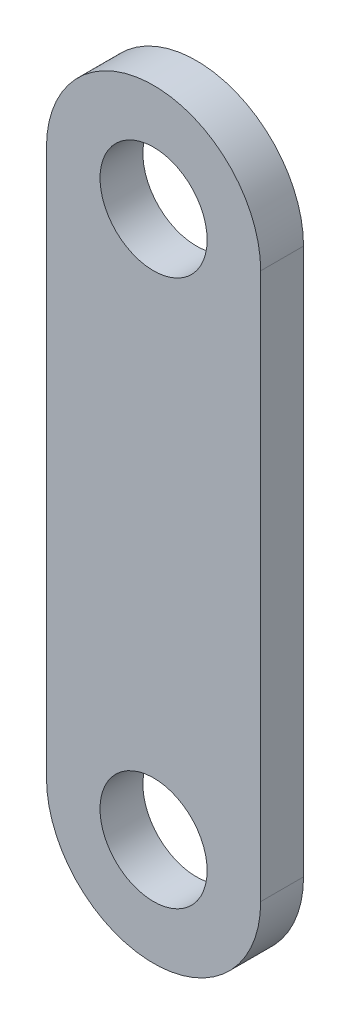
from build123d import *

# Parameters (mm, degrees)
LINK_BAR_PROFILE_R  = 25
LINK_BAR_20MM_DEPTH = 20


with BuildPart() as part:
    # Link Bar Profile → Link Bar 20mm (new body)
    with BuildSketch(Plane.XY):
        with BuildLine():
            Line((-50, 0), (-50, 255))
            ThreePointArc((-50, 255), (0, 305), (50, 255))
            Line((50, 255), (50, 0))
            ThreePointArc((50, 0), (0, -50), (-50, 0))
        make_face()
        with Locations((0, 255)):
            Circle(LINK_BAR_PROFILE_R, mode=Mode.SUBTRACT)
        Circle(LINK_BAR_PROFILE_R, mode=Mode.SUBTRACT)
    extrude(amount=LINK_BAR_20MM_DEPTH)


solid = part.part
